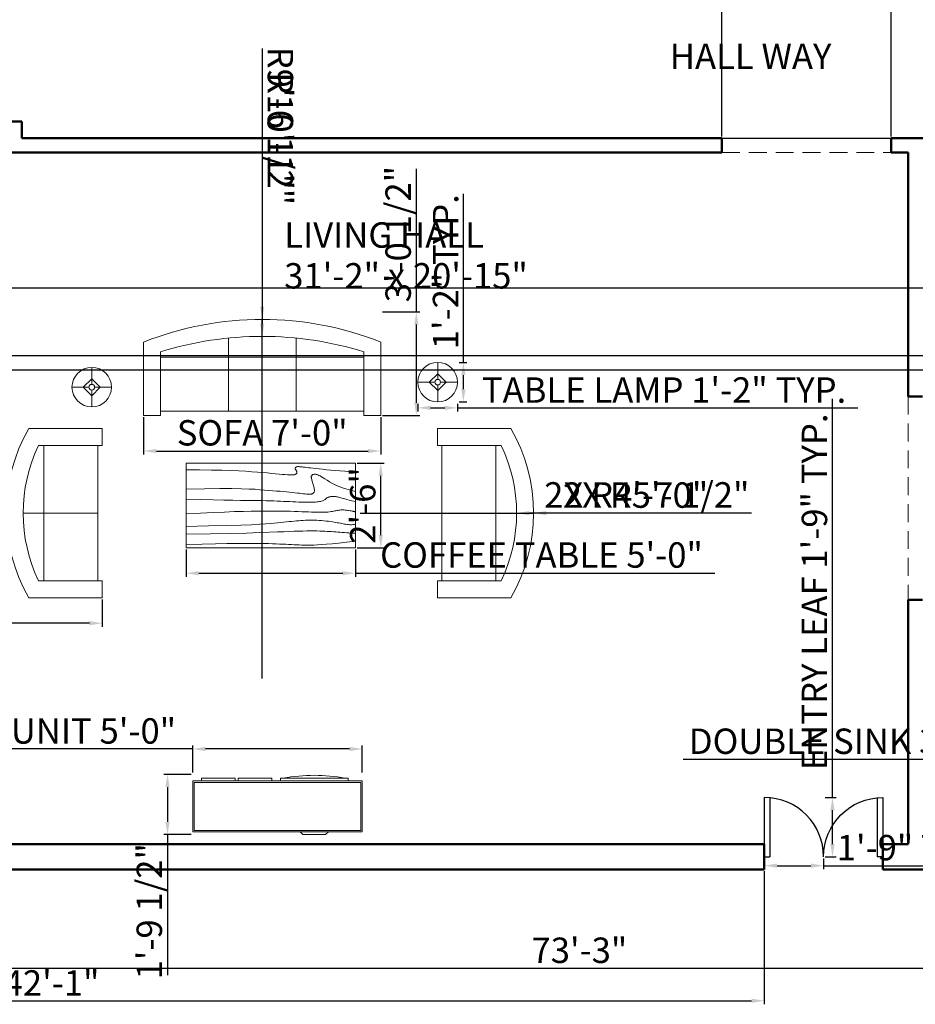
# Model space of a CAD drawing. Units: inches. Extents: x 2043 to 3102, y 1334 to 2053.
# Tile 2 of 4: x 2416 to 2734, y 1334 to 1683. Entities that reach past the tile are written whole.
import ezdxf

# ---------------------------------------------------------------- set-up
doc = ezdxf.new("R2010")
doc.units = ezdxf.units.IN
doc.linetypes.add('HIDDEN', pattern=[9.525, 6.35, -3.175])
for name, color, linetype, lineweight in [('A-ANNO-DIMS', 2, 'Continuous', 18), ('A-AREA-IDEN', 165, 'Continuous', 25), ('A-DOOR', 4, 'Continuous', 25), ('A-FURN', 8, 'Continuous', 18), ('A-WALL', 7, 'Continuous', 50), ('A-WALL-OVHD', 11, 'HIDDEN', 18)]:
    doc.layers.add(name, color=color, linetype=linetype, lineweight=lineweight)
doc.styles.get("Standard").update_dxf_attribs({"font": 'arial.ttf'})
doc.dimstyles.new('ISO-25', dxfattribs={"dimtxt": 9, "dimasz": 4.5, "dimexe": 1.25, "dimexo": 0.625, "dimtad": 1, "dimdec": 0, "dimlunit": 3, "dimtxsty": 'Standard', "dimcen": 2.5, "dimadec": 0, "dimazin": 0, "dimtfac": 1, "dimtdec": 0, "dimtmove": 0, "dimatfit": 3, "dimfxl": 1, "dimarcsym": 0})

# ---------------------------------------------------------------- blocks, each defined once
blk = doc.blocks.new('Table - Rectangular Woodgrain 60 x 30 in.')
for p, q in [((0, 0), (0, -30)), ((60, 0), (0, 0)), ((60, -30), (60, 0)), ((0, -30), (60, -30))]:
    blk.add_line(p, q)
for points in [[(0, -2.4), (4.8155, -2.418), (9.0302, -2.4688), (12.709, -2.5477), (15.9167, -2.65), (18.7181, -2.7711), (21.1781, -2.9063), (23.3616, -3.0508), (25.3333, -3.2), (27.1477, -3.3495), (28.8172, -3.4958), (30.3437, -3.636), (31.7291, -3.7667), (32.9756, -3.8849), (34.0849, -3.9875), (35.059, -4.0714), (35.9, -4.1334), (36.6114, -4.1711), (37.2041, -4.1854), (37.6906, -4.1779), (38.0833, -4.15), (38.3948, -4.1034), (38.6375, -4.0396), (38.8239, -3.9602), (38.9666, -3.8667), (39.0764, -3.7608), (39.1573, -3.6448), (39.2116, -3.521), (39.2416, -3.3917), (39.2498, -3.2593), (39.2385, -3.1261), (39.21, -2.9944), (39.1666, -2.8667), (39.111, -2.7447), (39.0468, -2.6281), (38.978, -2.5163), (38.9083, -2.4083), (38.8418, -2.3035), (38.7823, -2.201), (38.7337, -2.1001), (38.7, -2), (38.6844, -1.9003), (38.6875, -1.8021), (38.7094, -1.707), (38.75, -1.6167), (38.8094, -1.5326), (38.8875, -1.4563), (38.9844, -1.3893), (39.1, -1.3333), (39.2351, -1.2896), (39.3937, -1.2583), (39.5804, -1.2396), (39.8, -1.2333), (40.057, -1.2396), (40.3562, -1.2583), (40.7023, -1.2896), (41.1, -1.3333), (41.5547, -1.3895), (42.0755, -1.4573), (42.6721, -1.5361), (43.3542, -1.625), (44.1316, -1.7233), (45.014, -1.8302), (46.0114, -1.9449), (47.1333, -2.0667), (48.3862, -2.1947), (49.7625, -2.3281), (51.2513, -2.4663), (52.8416, -2.6083), (54.5226, -2.7535), (56.2833, -2.9011), (58.1127, -3.0501), (60, -3.2)], [(0, -9.2), (6.5759, -9.0858), (11.9385, -9.0365), (16.2527, -9.0418), (19.6833, -9.0917), (22.3952, -9.1759), (24.5531, -9.2844), (26.322, -9.4069), (27.8666, -9.5333), (29.3241, -9.6553), (30.7203, -9.7719), (32.0532, -9.8837), (33.3208, -9.9917), (34.5213, -10.0965), (35.6526, -10.199), (36.7128, -10.2999), (37.7, -10.4), (38.6129, -10.4996), (39.4531, -10.5969), (40.223, -10.6895), (40.925, -10.775), (41.5613, -10.8512), (42.1344, -10.9156), (42.6465, -10.966), (43.1, -11), (43.4976, -11.0158), (43.8437, -11.0136), (44.143, -10.9942), (44.4, -10.9583), (44.6195, -10.9069), (44.8062, -10.8406), (44.9648, -10.7603), (45.1, -10.6667), (45.2155, -10.5598), (45.3114, -10.4365), (45.3871, -10.2929), (45.4416, -10.125), (45.4743, -9.929), (45.4844, -9.7011), (45.4709, -9.4371), (45.4333, -9.1333), (45.3716, -8.7883), (45.2896, -8.4104), (45.1919, -8.0107), (45.0833, -7.6), (44.9685, -7.1893), (44.8521, -6.7896), (44.7388, -6.4117), (44.6333, -6.0667), (44.54, -5.7628), (44.4614, -5.4979), (44.4001, -5.2675), (44.3583, -5.0667), (44.3384, -4.8909), (44.3427, -4.7354), (44.3736, -4.5956), (44.4333, -4.4667), (44.5236, -4.3453), (44.6427, -4.2333), (44.7884, -4.1339), (44.9583, -4.05), (45.1501, -3.9849), (45.3614, -3.9417), (45.59, -3.9234), (45.8333, -3.9333), (46.0915, -3.9749), (46.3734, -4.0531), (46.6906, -4.1736), (47.0542, -4.3417), (47.4756, -4.5629), (47.9661, -4.8427), (48.5372, -5.1866), (49.2, -5.6), (49.9676, -6.0844), (50.8594, -6.625), (51.8965, -7.2031), (53.1, -7.8), (54.491, -8.3969), (56.0906, -8.975), (57.9199, -9.5156), (60, -10)], [(0, -12.8), (5.1847, -12.9322), (9.6213, -13.0323), (13.3963, -13.1059), (16.5958, -13.1583), (19.3063, -13.1952), (21.614, -13.2219), (23.6054, -13.2439), (25.3666, -13.2667), (26.9728, -13.2947), (28.4531, -13.3281), (29.8256, -13.3663), (31.1083, -13.4083), (32.3191, -13.4535), (33.476, -13.501), (34.597, -13.5501), (35.7, -13.6), (36.7984, -13.6497), (37.8875, -13.6979), (38.9578, -13.743), (40, -13.7833), (41.0047, -13.8174), (41.9625, -13.8438), (42.864, -13.8607), (43.7, -13.8667), (44.4631, -13.8604), (45.1552, -13.8417), (45.7801, -13.8104), (46.3416, -13.7667), (46.8439, -13.7104), (47.2906, -13.6417), (47.6858, -13.5604), (48.0333, -13.4667), (48.3375, -13.3608), (48.6042, -13.2448), (48.8396, -13.121), (49.05, -12.9917), (49.2417, -12.8593), (49.4208, -12.7261), (49.5937, -12.5944), (49.7667, -12.4667), (49.9452, -12.3451), (50.1323, -12.2313), (50.3303, -12.1268), (50.5416, -12.0333), (50.7686, -11.9524), (51.0135, -11.8854), (51.2788, -11.8341), (51.5666, -11.8), (51.8785, -11.7843), (52.2116, -11.7865), (52.562, -11.8059), (52.926, -11.8417), (53.2998, -11.8931), (53.6795, -11.9594), (54.0614, -12.0397), (54.4416, -12.1333), (54.8223, -12.2401), (55.2293, -12.3625), (55.6942, -12.5037), (56.2489, -12.6667), (56.9251, -12.8547), (57.7545, -13.0708), (58.7689, -13.3182), (60, -13.6)], [(0, -18), (5.124, -17.7273), (9.6609, -17.5057), (13.6705, -17.3303), (17.2125, -17.1958), (20.3467, -17.0973), (23.1328, -17.0297), (25.6307, -16.9878), (27.9, -16.9667), (29.9928, -16.9617), (31.9302, -16.9703), (33.7254, -16.9907), (35.3917, -17.0208), (36.9423, -17.0588), (38.3906, -17.1026), (39.7499, -17.1503), (41.0333, -17.2), (42.2519, -17.2496), (43.4073, -17.2969), (44.4986, -17.3395), (45.525, -17.375), (46.4858, -17.4012), (47.3802, -17.4156), (48.2074, -17.416), (48.9667, -17.4), (49.6583, -17.3662), (50.2872, -17.3167), (50.8595, -17.2547), (51.3812, -17.1833), (51.8584, -17.1057), (52.2971, -17.025), (52.7034, -16.9443), (53.0833, -16.8667), (53.443, -16.7951), (53.789, -16.7313), (54.128, -16.6768), (54.4666, -16.6334), (54.8115, -16.6024), (55.1693, -16.5854), (55.5465, -16.5841), (55.95, -16.6), (56.3828, -16.6337), (56.8346, -16.6823), (57.2915, -16.7418), (57.7396, -16.8084), (58.165, -16.878), (58.5539, -16.9469), (58.8924, -17.0111), (59.1666, -17.0667), (59.3679, -17.1107), (59.5078, -17.1438), (59.6032, -17.1675), (59.6708, -17.1833), (59.7275, -17.193), (59.7901, -17.1979), (59.8753, -17.1998), (60, -17.2)], [(0, -22.4), (8.0098, -22.2501), (14.4094, -22.1011), (19.4168, -21.9535), (23.25, -21.8083), (26.1269, -21.6663), (28.2656, -21.5281), (29.884, -21.3947), (31.2, -21.2667), (32.3967, -21.1448), (33.5172, -21.0292), (34.5697, -20.9198), (35.5625, -20.8167), (36.5037, -20.7198), (37.4015, -20.6292), (38.2642, -20.5448), (39.1, -20.4667), (39.9164, -20.3951), (40.7187, -20.3313), (41.5117, -20.2768), (42.3, -20.2333), (43.0883, -20.2024), (43.8812, -20.1854), (44.6836, -20.1841), (45.5, -20.2), (46.3328, -20.234), (47.1747, -20.2844), (48.0163, -20.3488), (48.8479, -20.425), (49.66, -20.5106), (50.4429, -20.6031), (51.1872, -20.7004), (51.8833, -20.8), (52.5246, -20.8999), (53.1166, -20.9995), (53.6681, -21.0983), (54.1875, -21.1958), (54.6834, -21.2919), (55.1646, -21.3859), (55.6394, -21.4777), (56.1167, -21.5667), (56.6028, -21.6515), (57.0961, -21.7266), (57.5929, -21.7852), (58.0896, -21.8208), (58.5823, -21.8268), (59.0674, -21.7964), (59.5412, -21.723), (60, -21.6)], [(0, -25.2), (8.6355, -25.0504), (15.7026, -24.9031), (21.4049, -24.7606), (25.9458, -24.625), (29.529, -24.4988), (32.3578, -24.3844), (34.6359, -24.284), (36.5667, -24.2), (38.3213, -24.1341), (39.9417, -24.0854), (41.437, -24.0523), (42.8167, -24.0333), (44.0901, -24.0268), (45.2667, -24.0313), (46.3557, -24.0451), (47.3667, -24.0667), (48.309, -24.0947), (49.1928, -24.1287), (50.0284, -24.168), (50.826, -24.2125), (51.5959, -24.2617), (52.3483, -24.3151), (53.0935, -24.3725), (53.8417, -24.4334), (54.6009, -24.497), (55.3699, -24.561), (56.1454, -24.6226), (56.9239, -24.6792), (57.7021, -24.7279), (58.4764, -24.7662), (59.2435, -24.7911), (60, -24.8)], [(0, -28.8), (5.6867, -28.6681), (10.45, -28.5698), (14.407, -28.5012), (17.675, -28.4584), (20.3711, -28.4374), (22.6125, -28.4344), (24.5164, -28.4455), (26.2, -28.4667), (27.762, -28.4947), (29.2276, -28.5281), (30.6033, -28.5663), (31.8958, -28.6084), (33.1118, -28.6535), (34.2578, -28.7011), (35.3405, -28.7501), (36.3666, -28.8), (37.3443, -28.8497), (38.288, -28.8974), (39.2137, -28.9412), (40.1375, -28.9792), (41.0753, -29.0093), (42.0432, -29.0297), (43.0572, -29.0384), (44.1333, -29.0333), (45.2936, -29.0114), (46.5843, -28.9641), (48.0579, -28.8816), (49.7666, -28.7542), (51.7629, -28.5721), (54.0989, -28.3255), (56.8272, -28.0048), (60, -27.6)]]:
    blk.add_lwpolyline(points)
blk = doc.blocks.new('Sofa - Roundback Loveseat 5 ft.')
for p, q in [((0, -32.44198), (0, -5.99998)), ((-24, -33.99998), (-24, -11.46958)), ((-23.9998, -13.38178), (23.99986, -13.38178)), ((24.00004, -33.99998), (24.00004, -11.46958)), ((-24, -32.44198), (24.00004, -32.44198))]:
    blk.add_line(p, q)
for points in [[(-24, -33.99998), (-30, -33.99998), (-30, -7.99998)], [(30.00004, -7.99998), (30.00004, -33.99998), (24.00004, -33.99998)]]:
    blk.add_lwpolyline(points)
for centre, radius, start, end in [((0, -60.24998), 60.24998, 60.13715, 119.8628), ((0, -61.38438), 55.38444, 64.32083, 115.6792)]:
    blk.add_arc(centre, radius, start, end)
blk = doc.blocks.new('Entertainment Center')
for p, q in [((-4, 0), (-5, -1)), ((4, 0), (-4, 0)), ((5, -1), (4, 0)), ((-17, -19), (-17, -1)), ((-17, -1), (43, -1)), ((-16.5, -18.5), (-16.5, -1.5)), ((-16.5, -1.5), (42.5, -1.5)), ((42.5, -1.5), (42.5, -18.5)), ((43, -1), (43, -19)), ((43, -19), (-17, -19)), ((42.5, -18.5), (-16.5, -18.5)), ((-12, -20), (-12, -19)), ((12, -20), (-12, -20)), ((12, -19), (12, -20)), ((15, -20), (15, -19)), ((27, -20), (15, -20)), ((27, -19), (27, -20)), ((28, -20), (28, -19)), ((40, -20), (28, -20)), ((40, -19), (40, -20))]:
    blk.add_line(p, q)
blk.add_arc((0, 40), 61, 259.6111, 280.3889)
blk = doc.blocks.new('Sofa - Roundback 7 ft.')
for p, q in [((-12.00002, -32.4421), (-12.00003, -6.5971)), ((11.99997, -32.4421), (11.99998, -6.5971)), ((-36.000027, -34), (-36.000027, -11.4696)), ((-35.999844, -13.3819), (35.9998, -13.3819)), ((35.99998, -34), (35.99998, -11.4696)), ((-36.000027, -32.4421), (35.99998, -32.4421))]:
    blk.add_line(p, q)
for points in [[(-36.000027, -34), (-42.000027, -34), (-42.000027, -8)], [(41.99998, -8), (41.99998, -34), (35.99998, -34)]]:
    blk.add_lwpolyline(points)
for centre, radius, start, end in [((0, -114.25), 114.25, 68.43141, 111.5686), ((-0.00001, -127.1968), 121.1968, 72.72033, 107.2797)]:
    blk.add_arc(centre, radius, start, end)
blk = doc.blocks.new('Lamp - Table')
for p, q in [((0, 7), (0, 1)), ((-1, 0), (-7, 0)), ((0, 3), (-3, 0)), ((-3, 0), (0, -3)), ((3, 0), (0, 3)), ((0, -3), (3, 0)), ((1, 0), (7, 0)), ((0, -1), (0, -7))]:
    blk.add_line(p, q)
for radius in [7, 1]:
    blk.add_circle((0, 0), radius)
blk = doc.blocks.new('*D20')
at = {"layer": 'A-ANNO-DIMS', "color": 0, "lineweight": -2, "transparency": 16777216}
for p, q in [((2175.19, 1381.63), (2175.19, 1346)), ((3054.19, 1381.63), (3054.19, 1346)), ((2179.69, 1347.25), (3049.69, 1347.25))]:
    blk.add_line(p, q, dxfattribs=at)
at = {"layer": 'A-ANNO-DIMS', "color": 0, "transparency": 16777216}
for points in [[(2179.69, 1348), (2179.69, 1346.5), (2175.19, 1347.25)], [(3049.69, 1348), (3049.69, 1346.5), (3054.19, 1347.25)]]:
    blk.add_solid(points, dxfattribs=at)
at = {"layer": 'Defpoints', "color": 0, "transparency": 16777216}
for p in [(2175.19, 1382.25), (3054.19, 1382.25), (3054.19, 1347.25)]:
    blk.add_point(p, dxfattribs=at)
at = {"layer": 'A-ANNO-DIMS', "color": 0, "transparency": 16777216, "insert": (2614.69, 1352.47), "char_height": 9, "attachment_point": 5}
blk.add_mtext('73\'-3"', dxfattribs=at)
blk = doc.blocks.new('DOOR-ENTRY-LEAF-21IN')
for p, q in [((0, 21), (0, 0)), ((2, 21), (2, 0)), ((0, 0), (2, 0))]:
    blk.add_line(p, q)
blk.add_arc((0, 0), 21, 0, 90)
blk = doc.blocks.new('*D38')
at = {"layer": 'A-ANNO-DIMS', "color": 0, "lineweight": -2, "transparency": 16777216}
for p, q in [((2704.34, 1407.75), (2704.34, 1548.93)), ((2701.81, 1407.75), (2705.59, 1407.75)), ((2704.34, 1391.25), (2704.34, 1403.25)), ((2701.81, 1386.75), (2705.59, 1386.75))]:
    blk.add_line(p, q, dxfattribs=at)
at = {"layer": 'A-ANNO-DIMS', "color": 0, "transparency": 16777216}
for points in [[(2703.59, 1403.25), (2705.09, 1403.25), (2704.34, 1407.75)], [(2703.59, 1391.25), (2705.09, 1391.25), (2704.34, 1386.75)]]:
    blk.add_solid(points, dxfattribs=at)
at = {"layer": 'Defpoints', "color": 0, "transparency": 16777216}
for p in [(2701.19, 1407.75), (2704.34, 1407.75), (2701.19, 1386.75)]:
    blk.add_point(p, dxfattribs=at)
at = {"layer": 'A-ANNO-DIMS', "color": 0, "transparency": 16777216, "insert": (2699.12, 1480.59), "char_height": 9, "attachment_point": 5, "rotation": 90}
blk.add_mtext('ENTRY LEAF 1\'-9" TYP.', dxfattribs=at)
blk = doc.blocks.new('*D39')
at = {"layer": 'A-ANNO-DIMS', "color": 0, "lineweight": -2, "transparency": 16777216}
for p, q in [((2680.19, 1386.13), (2680.19, 1382.35)), ((2701.19, 1386.13), (2701.19, 1382.35)), ((2684.69, 1383.6), (2696.69, 1383.6)), ((2701.19, 1383.6), (2760.95, 1383.6))]:
    blk.add_line(p, q, dxfattribs=at)
at = {"layer": 'A-ANNO-DIMS', "color": 0, "transparency": 16777216}
for points in [[(2684.69, 1384.35), (2684.69, 1382.85), (2680.19, 1383.6)], [(2696.69, 1384.35), (2696.69, 1382.85), (2701.19, 1383.6)]]:
    blk.add_solid(points, dxfattribs=at)
at = {"layer": 'Defpoints', "color": 0, "transparency": 16777216}
for p in [(2680.19, 1386.75), (2701.19, 1386.75), (2701.19, 1383.6)]:
    blk.add_point(p, dxfattribs=at)
at = {"layer": 'A-ANNO-DIMS', "color": 0, "transparency": 16777216, "insert": (2733.32, 1388.82), "char_height": 9, "attachment_point": 5}
blk.add_mtext('1\'-9" TYP.', dxfattribs=at)
blk = doc.blocks.new('*D41')
at = {"layer": 'A-ANNO-DIMS', "color": 0, "lineweight": -2, "transparency": 16777216}
for p, q in [((2408.96, 1477.85), (2408.96, 1468.23)), ((2445.63, 1477.85), (2445.63, 1468.23)), ((2408.96, 1469.48), (2327.39, 1469.48)), ((2441.13, 1469.48), (2413.46, 1469.48))]:
    blk.add_line(p, q, dxfattribs=at)
at = {"layer": 'A-ANNO-DIMS', "color": 0, "transparency": 16777216}
for points in [[(2413.46, 1470.23), (2413.46, 1468.73), (2408.96, 1469.48)], [(2441.13, 1470.23), (2441.13, 1468.73), (2445.63, 1469.48)]]:
    blk.add_solid(points, dxfattribs=at)
at = {"layer": 'Defpoints', "color": 0, "transparency": 16777216}
for p in [(2408.96, 1478.48), (2445.63, 1478.48), (2408.96, 1469.48)]:
    blk.add_point(p, dxfattribs=at)
at = {"layer": 'A-ANNO-DIMS', "color": 0, "transparency": 16777216, "insert": (2365.92, 1474.76), "char_height": 9, "attachment_point": 5}
blk.add_mtext('3\'-0 1/2" TYP.', dxfattribs=at)
blk = doc.blocks.new('*D42')
at = {"layer": 'A-ANNO-DIMS', "color": 0, "lineweight": -2, "transparency": 16777216}
for p, q in [((2557.48, 1547.24), (2557.48, 1544.51)), ((2561.98, 1545.76), (2566.98, 1545.76)), ((2571.48, 1547.24), (2571.48, 1544.51)), ((2571.48, 1545.76), (2713.37, 1545.76))]:
    blk.add_line(p, q, dxfattribs=at)
at = {"layer": 'A-ANNO-DIMS', "color": 0, "transparency": 16777216}
for points in [[(2561.98, 1546.51), (2561.98, 1545.01), (2557.48, 1545.76)], [(2566.98, 1546.51), (2566.98, 1545.01), (2571.48, 1545.76)]]:
    blk.add_solid(points, dxfattribs=at)
at = {"layer": 'Defpoints', "color": 0, "transparency": 16777216}
for p in [(2557.48, 1547.86), (2571.48, 1547.86), (2571.48, 1545.76)]:
    blk.add_point(p, dxfattribs=at)
at = {"layer": 'A-ANNO-DIMS', "color": 0, "transparency": 16777216, "insert": (2644.67, 1550.91), "char_height": 9, "attachment_point": 5}
blk.add_mtext('TABLE LAMP 1\'-2" TYP.', dxfattribs=at)
blk = doc.blocks.new('*D43')
at = {"layer": 'A-ANNO-DIMS', "color": 0, "lineweight": -2, "transparency": 16777216}
for p, q in [((2573.58, 1561.86), (2573.58, 1621.62)), ((2572.1, 1561.86), (2574.83, 1561.86)), ((2573.58, 1552.36), (2573.58, 1557.36)), ((2572.1, 1547.86), (2574.83, 1547.86))]:
    blk.add_line(p, q, dxfattribs=at)
at = {"layer": 'A-ANNO-DIMS', "color": 0, "transparency": 16777216}
for points in [[(2572.83, 1557.36), (2574.33, 1557.36), (2573.58, 1561.86)], [(2572.83, 1552.36), (2574.33, 1552.36), (2573.58, 1547.86)]]:
    blk.add_solid(points, dxfattribs=at)
at = {"layer": 'Defpoints', "color": 0, "transparency": 16777216}
for p in [(2571.48, 1561.86), (2573.58, 1561.86), (2571.48, 1547.86)]:
    blk.add_point(p, dxfattribs=at)
at = {"layer": 'A-ANNO-DIMS', "color": 0, "transparency": 16777216, "insert": (2568.43, 1593.99), "char_height": 9, "attachment_point": 5, "rotation": 90}
blk.add_mtext('1\'-2" TYP.', dxfattribs=at)
blk = doc.blocks.new('*D46')
at = {"layer": 'A-ANNO-DIMS', "color": 0, "lineweight": -2, "transparency": 16777216}
for p, q in [((2475.32, 1495.56), (2475.32, 1485.94)), ((2535.32, 1495.56), (2535.32, 1485.94)), ((2479.82, 1487.19), (2530.82, 1487.19)), ((2535.32, 1487.19), (2662.7, 1487.19))]:
    blk.add_line(p, q, dxfattribs=at)
at = {"layer": 'A-ANNO-DIMS', "color": 0, "transparency": 16777216}
for points in [[(2479.82, 1487.94), (2479.82, 1486.44), (2475.32, 1487.19)], [(2530.82, 1487.94), (2530.82, 1486.44), (2535.32, 1487.19)]]:
    blk.add_solid(points, dxfattribs=at)
at = {"layer": 'Defpoints', "color": 0, "transparency": 16777216}
for p in [(2475.32, 1496.19), (2535.32, 1496.19), (2535.32, 1487.19)]:
    blk.add_point(p, dxfattribs=at)
at = {"layer": 'A-ANNO-DIMS', "color": 0, "transparency": 16777216, "insert": (2601.26, 1492.47), "char_height": 9, "attachment_point": 5}
blk.add_mtext('COFFEE TABLE 5\'-0"', dxfattribs=at)
blk = doc.blocks.new('*D47')
at = {"layer": 'A-ANNO-DIMS', "color": 0, "lineweight": -2, "transparency": 16777216}
for p, q in [((2535.95, 1526.19), (2545.57, 1526.19)), ((2544.32, 1500.69), (2544.32, 1521.69)), ((2535.95, 1496.19), (2545.57, 1496.19))]:
    blk.add_line(p, q, dxfattribs=at)
at = {"layer": 'A-ANNO-DIMS', "color": 0, "transparency": 16777216}
for points in [[(2543.57, 1521.69), (2545.07, 1521.69), (2544.32, 1526.19)], [(2543.57, 1500.69), (2545.07, 1500.69), (2544.32, 1496.19)]]:
    blk.add_solid(points, dxfattribs=at)
at = {"layer": 'Defpoints', "color": 0, "transparency": 16777216}
for p in [(2535.32, 1526.19), (2544.32, 1526.19), (2535.32, 1496.19)]:
    blk.add_point(p, dxfattribs=at)
at = {"layer": 'A-ANNO-DIMS', "color": 0, "transparency": 16777216, "insert": (2539.1, 1511.19), "char_height": 9, "attachment_point": 5, "rotation": 90}
blk.add_mtext('2\'-6"', dxfattribs=at)
blk = doc.blocks.new('*D48')
at = {"layer": 'A-ANNO-DIMS', "color": 0, "lineweight": -2, "transparency": 16777216}
for p, q in [((2477.76, 1424.93), (2372.36, 1424.93)), ((2477.76, 1416.56), (2477.76, 1426.18)), ((2533.26, 1424.93), (2482.26, 1424.93)), ((2537.76, 1416.56), (2537.76, 1426.18))]:
    blk.add_line(p, q, dxfattribs=at)
at = {"layer": 'A-ANNO-DIMS', "color": 0, "transparency": 16777216}
for points in [[(2482.26, 1425.68), (2482.26, 1424.18), (2477.76, 1424.93)], [(2533.26, 1425.68), (2533.26, 1424.18), (2537.76, 1424.93)]]:
    blk.add_solid(points, dxfattribs=at)
at = {"layer": 'Defpoints', "color": 0, "transparency": 16777216}
for p in [(2477.76, 1424.93), (2477.76, 1415.93), (2537.76, 1415.93)]:
    blk.add_point(p, dxfattribs=at)
at = {"layer": 'A-ANNO-DIMS', "color": 0, "transparency": 16777216, "insert": (2422.81, 1430.15), "char_height": 9, "attachment_point": 5}
blk.add_mtext('MEDIA UNIT 5\'-0"', dxfattribs=at)
blk = doc.blocks.new('*D49')
at = {"layer": 'A-ANNO-DIMS', "color": 0, "lineweight": -2, "transparency": 16777216}
for p, q in [((2477.13, 1415.93), (2467.51, 1415.93)), ((2468.76, 1411.43), (2468.76, 1399.1)), ((2477.13, 1394.6), (2467.51, 1394.6)), ((2468.76, 1394.6), (2468.76, 1344.8))]:
    blk.add_line(p, q, dxfattribs=at)
at = {"layer": 'A-ANNO-DIMS', "color": 0, "transparency": 16777216}
for points in [[(2468.01, 1411.43), (2469.51, 1411.43), (2468.76, 1415.93)], [(2468.01, 1399.1), (2469.51, 1399.1), (2468.76, 1394.6)]]:
    blk.add_solid(points, dxfattribs=at)
at = {"layer": 'Defpoints', "color": 0, "transparency": 16777216}
for p in [(2477.76, 1415.93), (2468.76, 1394.6), (2477.76, 1394.6)]:
    blk.add_point(p, dxfattribs=at)
at = {"layer": 'A-ANNO-DIMS', "color": 0, "transparency": 16777216, "insert": (2463.48, 1367.45), "char_height": 9, "attachment_point": 5, "rotation": 90}
blk.add_mtext('1\'-9 1/2"', dxfattribs=at)
blk = doc.blocks.new('*D50')
at = {"layer": 'A-ANNO-DIMS', "color": 0, "lineweight": -2, "transparency": 16777216}
for p, q in [((2460.32, 1542.45), (2460.32, 1529.23)), ((2544.32, 1542.45), (2544.32, 1529.23)), ((2464.82, 1530.48), (2539.82, 1530.48))]:
    blk.add_line(p, q, dxfattribs=at)
at = {"layer": 'A-ANNO-DIMS', "color": 0, "transparency": 16777216}
for points in [[(2464.82, 1531.23), (2464.82, 1529.73), (2460.32, 1530.48)], [(2539.82, 1531.23), (2539.82, 1529.73), (2544.32, 1530.48)]]:
    blk.add_solid(points, dxfattribs=at)
at = {"layer": 'Defpoints', "color": 0, "transparency": 16777216}
for p in [(2460.32, 1543.08), (2544.32, 1543.08), (2544.32, 1530.48)]:
    blk.add_point(p, dxfattribs=at)
at = {"layer": 'A-ANNO-DIMS', "color": 0, "transparency": 16777216, "insert": (2502.32, 1535.76), "char_height": 9, "attachment_point": 5}
blk.add_mtext('SOFA 7\'-0"', dxfattribs=at)
blk = doc.blocks.new('*D51')
at = {"layer": 'A-ANNO-DIMS', "color": 0, "lineweight": -2, "transparency": 16777216}
for p, q in [((2556.92, 1579.74), (2556.92, 1630.38)), ((2544.95, 1579.74), (2558.17, 1579.74)), ((2556.92, 1547.58), (2556.92, 1575.24)), ((2544.95, 1543.08), (2558.17, 1543.08))]:
    blk.add_line(p, q, dxfattribs=at)
at = {"layer": 'A-ANNO-DIMS', "color": 0, "transparency": 16777216}
for points in [[(2556.17, 1575.24), (2557.67, 1575.24), (2556.92, 1579.74)], [(2556.17, 1547.58), (2557.67, 1547.58), (2556.92, 1543.08)]]:
    blk.add_solid(points, dxfattribs=at)
at = {"layer": 'Defpoints', "color": 0, "transparency": 16777216}
for p in [(2544.32, 1579.74), (2556.92, 1579.74), (2544.32, 1543.08)]:
    blk.add_point(p, dxfattribs=at)
at = {"layer": 'A-ANNO-DIMS', "color": 0, "transparency": 16777216, "insert": (2551.64, 1607.31), "char_height": 9, "attachment_point": 5, "rotation": 90}
blk.add_mtext('3\'-0 1/2"', dxfattribs=at)
blk = doc.blocks.new('*D58')
at = {"layer": 'A-ANNO-DIMS', "color": 0, "lineweight": -2, "transparency": 16777216}
for p, q in [((2768.68, 1421.23), (2651.42, 1421.23)), ((2768.68, 1416.46), (2768.68, 1422.48)), ((2800.18, 1421.23), (2773.18, 1421.23)), ((2804.68, 1416.46), (2804.68, 1422.48))]:
    blk.add_line(p, q, dxfattribs=at)
at = {"layer": 'A-ANNO-DIMS', "color": 0, "transparency": 16777216}
for points in [[(2773.18, 1421.98), (2773.18, 1420.48), (2768.68, 1421.23)], [(2800.18, 1421.98), (2800.18, 1420.48), (2804.68, 1421.23)]]:
    blk.add_solid(points, dxfattribs=at)
at = {"layer": 'Defpoints', "color": 0, "transparency": 16777216}
for p in [(2768.68, 1421.23), (2768.68, 1415.83), (2804.68, 1415.83)]:
    blk.add_point(p, dxfattribs=at)
at = {"layer": 'A-ANNO-DIMS', "color": 0, "transparency": 16777216, "insert": (2707.8, 1426.51), "char_height": 9, "attachment_point": 5}
blk.add_mtext('DOUBLE SINK 3\'-0"', dxfattribs=at)
blk = doc.blocks.new('*D60')
at = {"layer": 'A-ANNO-DIMS', "color": 0, "lineweight": -2, "transparency": 16777216}
for p, q in [((2423.81, 1697.25), (3101.95, 1697.25)), ((3100.7, 1645.75), (3100.7, 1692.75)), ((2417.81, 1641.25), (3101.95, 1641.25))]:
    blk.add_line(p, q, dxfattribs=at)
at = {"layer": 'A-ANNO-DIMS', "color": 0, "transparency": 16777216}
for points in [[(3099.95, 1692.75), (3101.45, 1692.75), (3100.7, 1697.25)], [(3099.95, 1645.75), (3101.45, 1645.75), (3100.7, 1641.25)]]:
    blk.add_solid(points, dxfattribs=at)
at = {"layer": 'Defpoints', "color": 0, "transparency": 16777216}
for p in [(2423.19, 1697.25), (3100.7, 1697.25), (2417.19, 1641.25)]:
    blk.add_point(p, dxfattribs=at)
at = {"layer": 'A-ANNO-DIMS', "color": 0, "transparency": 16777216, "insert": (3095.48, 1669.25), "char_height": 9, "attachment_point": 5, "rotation": 90}
blk.add_mtext('4\'-8"', dxfattribs=at)
blk = doc.blocks.new('*D62')
at = {"layer": 'A-ANNO-DIMS', "color": 0, "lineweight": -2, "transparency": 16777216}
for p, q in [((3100.7, 1588.25), (3100.7, 1618.08)), ((2352.81, 1588.25), (3101.95, 1588.25)), ((3100.7, 1568.75), (3100.7, 1583.75)), ((2352.81, 1564.25), (3101.95, 1564.25))]:
    blk.add_line(p, q, dxfattribs=at)
at = {"layer": 'A-ANNO-DIMS', "color": 0, "transparency": 16777216}
for points in [[(3099.95, 1583.75), (3101.45, 1583.75), (3100.7, 1588.25)], [(3099.95, 1568.75), (3101.45, 1568.75), (3100.7, 1564.25)]]:
    blk.add_solid(points, dxfattribs=at)
at = {"layer": 'Defpoints', "color": 0, "transparency": 16777216}
for p in [(2352.19, 1588.25), (3100.7, 1588.25), (2352.19, 1564.25)]:
    blk.add_point(p, dxfattribs=at)
at = {"layer": 'A-ANNO-DIMS', "color": 0, "transparency": 16777216, "insert": (3095.48, 1605.42), "char_height": 9, "attachment_point": 5, "rotation": 90}
blk.add_mtext('2\'-0"', dxfattribs=at)
blk = doc.blocks.new('*D64')
at = {"layer": 'A-ANNO-DIMS', "color": 0, "lineweight": -2, "transparency": 16777216}
for p, q in [((3100.7, 1568.75), (3100.7, 1573.25)), ((2352.81, 1564.25), (3101.95, 1564.25)), ((3100.7, 1564.25), (3100.7, 1559.25)), ((2352.81, 1559.25), (3101.95, 1559.25)), ((3100.7, 1554.75), (3100.7, 1525.08))]:
    blk.add_line(p, q, dxfattribs=at)
at = {"layer": 'A-ANNO-DIMS', "color": 0, "transparency": 16777216}
for points in [[(3099.95, 1568.75), (3101.45, 1568.75), (3100.7, 1564.25)], [(3099.95, 1554.75), (3101.45, 1554.75), (3100.7, 1559.25)]]:
    blk.add_solid(points, dxfattribs=at)
at = {"layer": 'Defpoints', "color": 0, "transparency": 16777216}
for p in [(2352.19, 1564.25), (2352.19, 1559.25), (3100.7, 1559.25)]:
    blk.add_point(p, dxfattribs=at)
at = {"layer": 'A-ANNO-DIMS', "color": 0, "transparency": 16777216, "insert": (3095.48, 1537.67), "char_height": 9, "attachment_point": 5, "rotation": 90}
blk.add_mtext('0\'-5"', dxfattribs=at)
blk = doc.blocks.new('*D66')
at = {"layer": 'A-ANNO-DIMS', "color": 0, "lineweight": -2, "transparency": 16777216}
for p, q in [((2664.56, 1636.25), (2127.43, 1636.25)), ((2128.68, 1395.75), (2128.68, 1631.75)), ((2679.56, 1391.25), (2127.43, 1391.25))]:
    blk.add_line(p, q, dxfattribs=at)
at = {"layer": 'A-ANNO-DIMS', "color": 0, "transparency": 16777216}
for points in [[(2127.93, 1631.75), (2129.43, 1631.75), (2128.68, 1636.25)], [(2127.93, 1395.75), (2129.43, 1395.75), (2128.68, 1391.25)]]:
    blk.add_solid(points, dxfattribs=at)
at = {"layer": 'Defpoints', "color": 0, "transparency": 16777216}
for p in [(2128.68, 1636.25), (2665.19, 1636.25), (2680.19, 1391.25)]:
    blk.add_point(p, dxfattribs=at)
at = {"layer": 'A-ANNO-DIMS', "color": 0, "transparency": 16777216, "insert": (2123.46, 1513.75), "char_height": 9, "attachment_point": 5, "rotation": 90}
blk.add_mtext('20\'-5"', dxfattribs=at)
blk = doc.blocks.new('*D67')
at = {"layer": 'A-ANNO-DIMS', "color": 0, "lineweight": -2, "transparency": 16777216}
for p, q in [((2665.19, 1641.88), (2665.19, 2024.01)), ((2725.19, 1641.88), (2725.19, 2024.01)), ((2669.69, 2022.76), (2720.69, 2022.76))]:
    blk.add_line(p, q, dxfattribs=at)
at = {"layer": 'A-ANNO-DIMS', "color": 0, "transparency": 16777216}
for points in [[(2669.69, 2023.51), (2669.69, 2022.01), (2665.19, 2022.76)], [(2720.69, 2023.51), (2720.69, 2022.01), (2725.19, 2022.76)]]:
    blk.add_solid(points, dxfattribs=at)
at = {"layer": 'Defpoints', "color": 0, "transparency": 16777216}
for p in [(2725.19, 2022.76), (2665.19, 1641.25), (2725.19, 1641.25)]:
    blk.add_point(p, dxfattribs=at)
at = {"layer": 'A-ANNO-DIMS', "color": 0, "transparency": 16777216, "insert": (2695.19, 2027.98), "char_height": 9, "attachment_point": 5}
blk.add_mtext('5\'-0"', dxfattribs=at)
blk = doc.blocks.new('*D68')
at = {"layer": 'A-ANNO-DIMS', "color": 0, "lineweight": -2, "transparency": 16777216}
for p, q in [((2175.19, 1381.63), (2175.19, 1334.49)), ((2680.19, 1381.63), (2680.19, 1334.49)), ((2179.69, 1335.74), (2675.69, 1335.74))]:
    blk.add_line(p, q, dxfattribs=at)
at = {"layer": 'A-ANNO-DIMS', "color": 0, "transparency": 16777216}
for points in [[(2179.69, 1336.49), (2179.69, 1334.99), (2175.19, 1335.74)], [(2675.69, 1336.49), (2675.69, 1334.99), (2680.19, 1335.74)]]:
    blk.add_solid(points, dxfattribs=at)
at = {"layer": 'Defpoints', "color": 0, "transparency": 16777216}
for p in [(2175.19, 1382.25), (2680.19, 1382.25), (2680.19, 1335.74)]:
    blk.add_point(p, dxfattribs=at)
at = {"layer": 'A-ANNO-DIMS', "color": 0, "transparency": 16777216, "insert": (2427.69, 1340.89), "char_height": 9, "attachment_point": 5}
blk.add_mtext('42\'-1"', dxfattribs=at)
blk = doc.blocks.new('*D69')
at = {"layer": 'A-ANNO-DIMS', "color": 0, "lineweight": -2, "transparency": 16777216}
for p, q in [((2502.32, 1664.18), (2502.32, 1575.58)), ((2502.32, 1449.88), (2502.32, 1571.08))]:
    blk.add_line(p, q, dxfattribs=at)
at = {"layer": 'A-ANNO-DIMS', "color": 0, "transparency": 16777216}
blk.add_solid([(2503.07, 1575.58), (2501.57, 1575.58), (2502.32, 1571.08)], dxfattribs=at)
at = {"layer": 'Defpoints', "color": 0, "transparency": 16777216}
for p in [(2502.32, 1571.08), (2502.32, 1449.88)]:
    blk.add_point(p, dxfattribs=at)
at = {"layer": 'A-ANNO-DIMS', "color": 0, "transparency": 16777216, "insert": (2507.54, 1643.79), "char_height": 9, "attachment_point": 5, "rotation": 270.0001}
blk.add_mtext('R10\'-1"', dxfattribs=at)
blk = doc.blocks.new('*D70')
at = {"layer": 'A-ANNO-DIMS', "color": 0, "lineweight": -2, "transparency": 16777216}
for p, q in [((2502.32, 1673), (2502.32, 1581.58)), ((2502.32, 1462.83), (2502.32, 1577.08))]:
    blk.add_line(p, q, dxfattribs=at)
at = {"layer": 'A-ANNO-DIMS', "color": 0, "transparency": 16777216}
blk.add_solid([(2503.07, 1581.58), (2501.57, 1581.58), (2502.32, 1577.08)], dxfattribs=at)
at = {"layer": 'Defpoints', "color": 0, "transparency": 16777216}
for p in [(2502.32, 1577.08), (2502.32, 1462.83)]:
    blk.add_point(p, dxfattribs=at)
at = {"layer": 'A-ANNO-DIMS', "color": 0, "transparency": 16777216, "insert": (2507.6, 1645.63), "char_height": 9, "attachment_point": 5, "rotation": 270.0002}
blk.add_mtext('R9\'-6 1/2"', dxfattribs=at)
blk = doc.blocks.new('*D71')
at = {"layer": 'A-ANNO-DIMS', "color": 0, "lineweight": -2, "transparency": 16777216}
for p, q in [((2538.19, 1508.48), (2598.44, 1508.48)), ((2661.23, 1508.48), (2602.94, 1508.48))]:
    blk.add_line(p, q, dxfattribs=at)
at = {"layer": 'A-ANNO-DIMS', "color": 0, "transparency": 16777216}
blk.add_solid([(2602.94, 1509.23), (2602.94, 1507.73), (2598.44, 1508.48)], dxfattribs=at)
at = {"layer": 'Defpoints', "color": 0, "transparency": 16777216}
for p in [(2538.19, 1508.48), (2598.44, 1508.48)]:
    blk.add_point(p, dxfattribs=at)
at = {"layer": 'A-ANNO-DIMS', "color": 0, "transparency": 16777216, "insert": (2634.59, 1513.7), "char_height": 9, "attachment_point": 5, "rotation": 359.9998}
blk.add_mtext('2X R5\'-0"', dxfattribs=at)
blk = doc.blocks.new('*D72')
at = {"layer": 'A-ANNO-DIMS', "color": 0, "lineweight": -2, "transparency": 16777216}
for p, q in [((2537.06, 1508.48), (2592.44, 1508.48)), ((2675.69, 1508.48), (2596.94, 1508.48))]:
    blk.add_line(p, q, dxfattribs=at)
at = {"layer": 'A-ANNO-DIMS', "color": 0, "transparency": 16777216}
blk.add_solid([(2596.94, 1509.23), (2596.94, 1507.73), (2592.44, 1508.48)], dxfattribs=at)
at = {"layer": 'Defpoints', "color": 0, "transparency": 16777216}
for p in [(2537.06, 1508.48), (2592.44, 1508.48)]:
    blk.add_point(p, dxfattribs=at)
at = {"layer": 'A-ANNO-DIMS', "color": 0, "transparency": 16777216, "insert": (2638.57, 1513.76), "char_height": 9, "attachment_point": 5, "rotation": 359.9998}
blk.add_mtext('2X R4\'-7 1/2"', dxfattribs=at)

msp = doc.modelspace()

# ---------------------------------------------------------------- linework, layer by layer
at = {"layer": 'A-WALL'}
for p, q in [((2412.19, 1647.25), (2417.19, 1647.25)), ((2417.19, 1647.25), (2417.19, 1641.25)), ((2417.19, 1641.25), (2665.19, 1641.25)), ((2665.19, 1641.25), (2665.19, 1636.25)), ((2725.19, 1641.25), (2725.19, 1636.25)), ((2725.19, 1641.25), (2812.19, 1641.25)), ((2261.19, 1636.25), (2665.19, 1636.25)), ((2725.19, 1636.25), (2731.19, 1636.25)), ((2731.19, 1636.25), (2731.19, 1549.75)), ((2736.19, 1549.75), (2731.19, 1549.75)), ((2736.19, 1477.75), (2731.19, 1477.75)), ((2731.19, 1477.75), (2731.19, 1391.25)), ((2357.19, 1391.25), (2680.19, 1391.25)), ((2680.19, 1391.25), (2680.19, 1382.25)), ((2722.19, 1391.25), (2722.19, 1382.25)), ((2722.19, 1391.25), (2731.19, 1391.25)), ((2175.19, 1382.25), (2680.19, 1382.25)), ((2722.19, 1382.25), (3054.19, 1382.25))]:
    msp.add_line(p, q, dxfattribs=at)
at = {"layer": 'A-WALL-OVHD'}
for p, q in [((2665.19, 1641.25), (2725.19, 1641.25)), ((2665.19, 1636.25), (2725.19, 1636.25)), ((2731.19, 1549.75), (2731.19, 1477.75))]:
    msp.add_line(p, q, dxfattribs=at)

# ---------------------------------------------------------------- block references
at = {"layer": 'A-DOOR'}
msp.add_blockref('DOOR-ENTRY-LEAF-21IN', (2680.19, 1386.76), dxfattribs=at)
at = {"layer": 'A-DOOR', "extrusion": (0, 0, -1), "zscale": -1}
msp.add_blockref('DOOR-ENTRY-LEAF-21IN', (-2722.19, 1386.76), dxfattribs=at)
at = {"layer": 'A-FURN'}
for name, p in [('Sofa - Roundback 7 ft.', (2502.32, 1577.08)), ('Lamp - Table', (2441.93, 1553.08)), ('Lamp - Table', (2564.48, 1554.86)), ('Table - Rectangular Woodgrain 60 x 30 in.', (2475.32, 1526.19))]:
    msp.add_blockref(name, p, dxfattribs=at)
for name, p, rotation in [('Sofa - Roundback Loveseat 5 ft.', (2411.63, 1508.48), 90), ('Sofa - Roundback Loveseat 5 ft.', (2598.44, 1508.48), 270), ('Entertainment Center', (2520.76, 1394.6), 180)]:
    msp.add_blockref(name, p, dxfattribs=dict(at, rotation=rotation))

# ---------------------------------------------------------------- texts
at = {"layer": 'A-AREA-IDEN'}
for s, p in [('HALL WAY', (2646.71, 1665.78)), ('LIVING HALL', (2510.12, 1602.49)), ('31\'-2" x 20\'-15"', (2510.12, 1588.03))]:
    msp.add_text(s, height=9, dxfattribs=at).set_placement(p)

# ---------------------------------------------------------------- dimensions: what is measured, and where the dimension line sits
at = {"layer": 'A-ANNO-DIMS'}
for base, p1, p2, override, picture, middle in [((2725.19, 2022.76), (2665.19, 1641.25), (2725.19, 1641.25), {"dimdec": 1, "dimlfac": 1, "dimrnd": 0, "dimzin": 1, "dimdsep": 46, "dimlunit": 4, "dimfrac": 2}, '*D67', (2695.19, 2027.98)), ((3054.19, 1347.25), (2175.19, 1382.25), (3054.19, 1382.25), {"dimclrd": 0, "dimclre": 0, "dimclrt": 0}, '*D20', (2614.69, 1352.47)), ((2680.19, 1335.74), (2175.19, 1382.25), (2680.19, 1382.25), {"dimdec": 1, "dimlfac": 1, "dimrnd": 0, "dimzin": 1, "dimdsep": 46, "dimlunit": 4, "dimfrac": 2}, '*D68', (2427.69, 1340.89))]:
    dim = msp.add_linear_dim(base=base, p1=p1, p2=p2, dimstyle='ISO-25', override=override, dxfattribs=at)
    dim.commit()
    dim.dimension.update_dxf_attribs({"geometry": picture, "text_midpoint": middle})
for base, p1, p2, angle, picture, middle in [((3100.7, 1697.25), (2417.19, 1641.25), (2423.19, 1697.25), 90, '*D60', (3095.48, 1669.25)), ((2128.68, 1636.25), (2680.19, 1391.25), (2665.19, 1636.25), 90, '*D66', (2123.46, 1513.75)), ((2556.92, 1579.74), (2544.32, 1543.08), (2544.32, 1579.74), 90, '*D51', (2551.64, 1607.31)), ((3100.7, 1588.25), (2352.19, 1564.25), (2352.19, 1588.25), 90, '*D62', (3095.48, 1605.42)), ((3100.7, 1559.25), (2352.19, 1564.25), (2352.19, 1559.25), 90, '*D64', (3095.48, 1537.67)), ((2544.32, 1526.19), (2535.32, 1496.19), (2535.32, 1526.19), 90, '*D47', (2539.1, 1511.19)), ((2468.76, 1394.6), (2477.76, 1415.93), (2477.76, 1394.6), 270, '*D49', (2463.48, 1367.45))]:
    dim = msp.add_linear_dim(base=base, p1=p1, p2=p2, angle=angle, dimstyle='ISO-25', override={"dimdec": 1, "dimlfac": 1, "dimrnd": 0, "dimzin": 1, "dimdsep": 46, "dimlunit": 4, "dimfrac": 2}, dxfattribs=at)
    dim.commit()
    dim.dimension.update_dxf_attribs({"geometry": picture, "text_midpoint": middle})
for center, mpoint, picture, middle in [((2502.321324, 1462.825241), (2502.321, 1577.075241), '*D70', (2502.3208056, 1645.625241)), ((2502.32, 1449.88), (2502.32, 1571.08), '*D69', (2502.32, 1643.79))]:
    dim = msp.add_radius_dim(center=center, mpoint=mpoint, dimstyle='ISO-25', override={"dimdec": 1, "dimlfac": 1, "dimrnd": 0, "dimzin": 1, "dimdsep": 46, "dimlunit": 4, "dimfrac": 2}, dxfattribs=at)
    dim.commit()
    dim.dimension.update_dxf_attribs({"geometry": picture, "text_midpoint": middle, "dimtype": 164})
for base, p1, p2, angle, text, picture, middle in [((2573.58, 1561.86), (2571.48, 1547.86), (2571.48, 1561.86), 90, '<> TYP.', '*D43', (2568.43, 1593.99)), ((2704.34, 1407.75), (2701.19, 1386.75), (2701.19, 1407.75), 90, 'ENTRY LEAF <> TYP.', '*D38', (2699.12, 1480.59)), ((2408.96, 1469.48), (2445.63, 1478.48), (2408.96, 1478.48), 180, '<> TYP.', '*D41', (2365.92, 1474.76)), ((2477.76, 1424.93), (2537.76, 1415.93), (2477.76, 1415.93), 180, 'MEDIA UNIT <>', '*D48', (2422.81, 1430.15)), ((2768.68, 1421.23), (2804.68, 1415.83), (2768.68, 1415.83), 180, 'DOUBLE SINK <>', '*D58', (2707.8, 1426.51))]:
    dim = msp.add_linear_dim(base=base, p1=p1, p2=p2, angle=angle, text=text, dimstyle='ISO-25', override={"dimdec": 1, "dimlfac": 1, "dimrnd": 0, "dimzin": 1, "dimdsep": 46, "dimlunit": 4, "dimfrac": 2}, dxfattribs=at)
    dim.commit()
    dim.dimension.update_dxf_attribs({"geometry": picture, "text_midpoint": middle})
for base, p1, p2, text, picture, middle in [((2571.48, 1545.76), (2557.48, 1547.86), (2571.48, 1547.86), 'TABLE LAMP <> TYP.', '*D42', (2644.67, 1550.91)), ((2544.32, 1530.48), (2460.32, 1543.08), (2544.32, 1543.08), 'SOFA <>', '*D50', (2502.32, 1535.76)), ((2535.32, 1487.19), (2475.32, 1496.19), (2535.32, 1496.19), 'COFFEE TABLE <>', '*D46', (2601.26, 1492.47)), ((2701.19, 1383.6), (2680.19, 1386.75), (2701.19, 1386.75), '<> TYP.', '*D39', (2733.32, 1388.82))]:
    dim = msp.add_linear_dim(base=base, p1=p1, p2=p2, text=text, dimstyle='ISO-25', override={"dimdec": 1, "dimlfac": 1, "dimrnd": 0, "dimzin": 1, "dimdsep": 46, "dimlunit": 4, "dimfrac": 2}, dxfattribs=at)
    dim.commit()
    dim.dimension.update_dxf_attribs({"geometry": picture, "text_midpoint": middle})
dim = msp.add_radius_dim(center=(2537.06, 1508.48), mpoint=(2592.44, 1508.48), text='2X <>', dimstyle='ISO-25', override={"dimdec": 1, "dimlfac": 1, "dimrnd": 0, "dimzin": 1, "dimdsep": 46, "dimlunit": 4, "dimfrac": 2}, dxfattribs=at)
dim.commit()
dim.dimension.update_dxf_attribs({"geometry": '*D72', "text_midpoint": (2638.57, 1513.76)})
dim = msp.add_radius_dim(center=(2538.1905, 1508.4782), mpoint=(2598.4404, 1508.478), text='2X <>', dimstyle='ISO-25', override={"dimdec": 1, "dimlfac": 1, "dimrnd": 0, "dimzin": 1, "dimdsep": 46, "dimlunit": 4, "dimfrac": 2}, dxfattribs=at)
dim.commit()
dim.dimension.update_dxf_attribs({"geometry": '*D71', "text_midpoint": (2634.5904, 1508.4779), "dimtype": 164})

doc.saveas('drawing.dxf')
